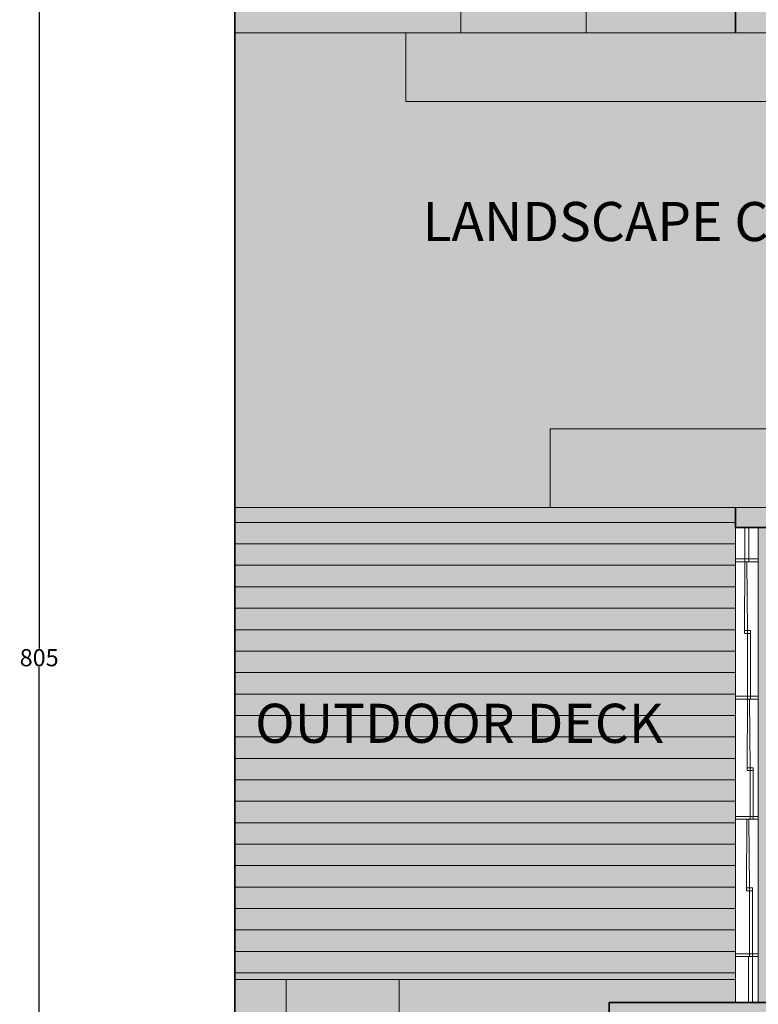
# Model space of a CAD drawing. Units: inches. Extents: x 1704 to 6393, y -157 to 1172.
# Tile 39 of 122: x 1823 to 2081, y 372 to 716. Entities that reach past the tile are written whole.
import ezdxf

# ---------------------------------------------------------------- set-up
doc = ezdxf.new("R2010")
doc.units = ezdxf.units.IN
doc.header["$MEASUREMENT"] = 0
for name, color, linetype, lineweight in [('A-ANNO-DIMS', 7, 'Continuous', 13), ('A-AREA-IDEN', 7, 'Continuous', 18), ('A-WALL-PATT', 7, 'Continuous', 13), ('C-PROP', 7, 'Continuous', 35), ('GLASS PANEL FASADE', 4, 'Continuous', 18), ('L-DECK-PLNK-PATT', 250, 'Continuous', 13), ('L-HRDS', 8, 'Continuous', 18), ('L-PVMT-PATT', 8, 'Continuous', 13), ('WALLS', 7, 'Continuous', 35)]:
    doc.layers.add(name, color=color, linetype=linetype, lineweight=lineweight)
for name, color, linetype, lineweight, true_color in [('A-FLOR-PATT', 7, 'Continuous', 13, 0xf2f2f2), ('L-DECK-PATT', 35, 'Continuous', 13, 0xa6725b), ('L-HRDS-PATT', 9, 'Continuous', 13, 0xc5c1ba), ('L-PLNT-PATT', 253, 'Continuous', 13, 0x9abc8f)]:
    doc.layers.add(name, color=color, linetype=linetype, lineweight=lineweight, true_color=true_color)
doc.styles.get("Standard").update_dxf_attribs({"font": 'arial.ttf'})
doc.dimstyles.get("Standard").update_dxf_attribs({"dimtxt": 6, "dimasz": 2, "dimexe": 0.18, "dimexo": 0.0625, "dimgap": 0.09, "dimtad": 0, "dimtih": 1, "dimtoh": 1, "dimdec": 1, "dimzin": 0, "dimdsep": 46, "dimlunit": 3, "dimtxsty": 'Standard', "dimblk": 'ARCHTICK', "dimcen": 0.09, "dimadec": 0, "dimazin": 0, "dimtfac": 1, "dimtdec": 1, "dimtofl": 0, "dimtmove": 0, "dimatfit": 3, "dimfxl": 1, "dimtolj": 1, "dimtzin": 0, "dimarcsym": 0})

# ---------------------------------------------------------------- blocks, each defined once
blk = doc.blocks.new('_ArchTick')
at = {"color": 0, "linetype": 'ByBlock', "const_width": 0.15}
blk.add_lwpolyline([(-0.5, -0.5), (0.5, 0.5)], dxfattribs=at)
blk = doc.blocks.new('*D93')
at = {"layer": 'A-ANNO-DIMS', "color": 0, "lineweight": -2, "transparency": 16777216}
for p, q in [((2605.29, 895.21), (1829.7, 895.21)), ((1829.88, 895.21), (1829.88, 495.87)), ((1829.88, 90.21), (1829.88, 489.56)), ((2605.29, 90.21), (1829.7, 90.21))]:
    blk.add_line(p, q, dxfattribs=at)
at = {"layer": 'Defpoints', "color": 0, "lineweight": -3, "transparency": 16777216}
for p in [(2605.35, 895.21), (1829.88, 90.21), (2605.35, 90.21)]:
    blk.add_point(p, dxfattribs=at)
at = {"layer": 'A-ANNO-DIMS', "color": 0, "lineweight": -2, "transparency": 16777216, "xscale": 2, "yscale": 2, "zscale": 2}
for p, rotation in [((1829.88, 895.21), 90), ((1829.88, 90.21), 270)]:
    blk.add_blockref('_ArchTick', p, dxfattribs=dict(at, rotation=rotation))
at = {"layer": 'A-ANNO-DIMS', "color": 0, "transparency": 16777216, "insert": (1829.88, 492.71), "char_height": 6, "attachment_point": 5}
blk.add_mtext('\\A1;805', dxfattribs=at)

msp = doc.modelspace()

# ---------------------------------------------------------------- hatches: boundary and pattern name
at = {"layer": 'A-FLOR-PATT', "transparency": 33554528}
h = msp.add_hatch(color=256, dxfattribs=at)
h.dxf.hatch_style = 1
h.paths.add_polyline_path([(2273.349, 538.213), (2081.349, 538.213), (2081.349, 372.213), (2273.349, 372.213)])
h.paths.add_polyline_path([(2189.542, 505.951), (2184.316, 505.951), (2184.316, 505.591), (2169.442, 505.591), (2169.442, 505.951), (2164.216, 505.951, -0.4142136), (2163.814, 506.353), (2163.814, 526.093, -0.4142136), (2164.216, 526.495), (2189.542, 526.495, -0.4142136), (2189.944, 526.093), (2189.944, 506.353, -0.4142136)], flags=16)
h.paths.add_polyline_path([(2200.535, 511.491), (2200.535, 526.191), (2217.621, 526.191), (2217.621, 511.491), (2214.605, 511.491, -0.3946213), (2214.203, 511.116), (2203.952, 511.116, -0.3946213), (2203.551, 511.491)], flags=16)
h.paths.add_polyline_path([(2200.736, 511.692), (2200.736, 525.99), (2203.55, 525.99), (2203.55, 523.838, 0.1045605), (2214.605, 523.838), (2214.605, 525.99), (2217.42, 525.99), (2217.42, 511.692), (2214.605, 511.692), (2214.605, 523.838, -0.1045605), (2203.55, 523.838), (2203.55, 511.692)], flags=0)
h.paths.add_polyline_path([(2203.952, 511.317, -0.4142136), (2203.751, 511.518), (2203.751, 523.591, 0.099912), (2214.404, 523.591), (2214.404, 511.518, -0.4142136), (2214.203, 511.317)], flags=0)
h.paths.add_polyline_path([(2184.084, 516.015, -0.0686795), (2169.674, 516.015), (2169.674, 522.073), (2184.084, 522.073)], flags=0)
h.paths.add_polyline_path([(2183.325, 518.606, -0.0772766), (2170.433, 518.606), (2170.433, 521.123, -0.0235462), (2183.325, 521.123)], flags=0)
h.paths.add_polyline_path([(2135.029, 507.225, -0.1405189), (2135.191, 507.834, -0.0513838), (2135.029, 507.797)], flags=16)
h.paths.add_polyline_path([(2146.318, 498.997, -0.0311848), (2144.279, 499.202, -0.1719602), (2141.865, 499.263, -0.2234326), (2139.482, 499.263, -0.1719602), (2137.068, 499.202, -0.0311848), (2135.029, 498.997, -0.066975), (2135.029, 505.313, -0.0276914), (2136.841, 505.144), (2136.841, 506.777), (2136.576, 506.777), (2136.576, 507.371, 0.039911), (2145.741, 507.448, 0.2546956), (2146.318, 507.225), (2146.318, 507.269, 0.1305786), (2146.156, 507.834, -0.0704067), (2145.953, 507.935, -0.011584), (2145.714, 508.002, -0.2546956), (2145.137, 507.779, -0.2546956), (2145.361, 508.355, -0.0259693), (2145.107, 516.407, -0.0070422), (2144.025, 516.297, -0.1828112), (2142.939, 516.218, -0.2042746), (2142.015, 516.175, -0.1805419), (2139.348, 516.174, -0.0000184), (2139.345, 516.174, -0.2035615), (2138.425, 516.217, -0.0000237), (2138.421, 516.217, -0.1818152), (2137.34, 516.296, -0.0071635), (2136.24, 516.407, 0.007166), (2136.162, 518.63, 0.314303), (2135.854, 518.974, -0.1253469), (2135.537, 518.935, -0.2546956), (2135.76, 519.512, -0.0162662), (2135.67, 519.849, -0.296972), (2135.535, 520.8, -0.227702), (2135.464, 521.698, 0.1283977), (2132.757, 521.718), (2132.757, 525.785, -0.4142136), (2133.331, 526.359), (2148.015, 526.359, -0.4142136), (2148.589, 525.785), (2148.589, 521.718, -0.0118936), (2148.835, 521.65, -0.2546956), (2149.412, 521.873, -0.2546956), (2149.188, 521.296, -0.0417628), (2149.188, 508.355, -0.2546956), (2149.412, 507.779, -0.2546956), (2148.835, 508.002, -0.011584), (2148.596, 507.935, -0.2124435), (2147.949, 507.813, -0.2363999), (2147.423, 507.772, -0.3143526), (2147.126, 507.772, -0.2363999), (2146.6, 507.813, -0.0879275), (2146.318, 507.797), (2146.318, 507.225, -0.2546956), (2145.741, 507.448, -0.0042329), (2144.771, 507.371), (2144.771, 506.777), (2144.506, 506.777), (2144.506, 505.144, -0.0276914), (2146.318, 505.313, -0.066975)], flags=16)
h.paths.add_polyline_path([(2141.865, 505.047, 0.2234326), (2139.482, 505.047, 0.1738145), (2137.043, 505.1), (2137.043, 506.317), (2137.335, 506.317), (2137.335, 505.184, -0.1522072), (2139.482, 505.047, -0.2234326), (2141.865, 505.047, -0.1522072), (2144.011, 505.184), (2144.011, 506.317), (2144.304, 506.317), (2144.304, 505.1, 0.1738145)], flags=0)
h.paths.add_polyline_path([(2145.233, 522.986, 0.0079197), (2144.017, 523.111, 0.1826165), (2142.931, 523.19, 0.2042746), (2142.008, 523.233, 0.1806536), (2139.339, 523.233, 0.2042746), (2138.415, 523.19, 0.1826165), (2137.33, 523.111, 0.0079197), (2136.114, 522.986, 0.1967082), (2135.679, 523.212, 0.047677), (2135.755, 524.004), (2134.638, 521.852), (2134.376, 524.691, -0.2583282), (2135.029, 526.359, -0.0890464), (2135.632, 525.01, -0.1830277), (2145.715, 525.01, -0.0890464), (2146.318, 526.359, -0.2583282), (2146.971, 524.691), (2146.709, 521.852), (2145.592, 524.004, 0.047677), (2145.668, 523.212, 0.1967082)], flags=0)
h.paths.add_polyline_path([(2144.419, 519.027, -0.0368796), (2136.927, 519.027, -0.0368796)], flags=0)
h.paths.add_polyline_path([(2273.349, 629.213), (2213.349, 629.213), (2213.349, 573.213), (2213.349, 545.213), (2273.349, 545.213)])
h.paths.add_polyline_path([(2273.349, 711.213), (2207.349, 711.213), (2207.349, 709.213), (2231.349, 709.213), (2231.349, 707.213), (2207.349, 707.213), (2207.349, 631.213), (2273.349, 631.213)])
h.paths.add_polyline_path([(2273.349, 364.213), (2081.349, 364.213), (2081.349, 202.213), (2225.349, 202.213), (2229.181, 202.213), (2230.482, 202.213), (2268.215, 202.213), (2269.516, 202.213), (2273.349, 202.213)])
h.paths.add_polyline_path([(2203.551, 339.558, 0.3946213), (2203.952, 339.183), (2214.203, 339.183), (2214.203, 339.384), (2203.751, 339.384), (2203.751, 339.558)], flags=16)
h.paths.add_polyline_path([(2203.55, 351.7), (2203.55, 339.759), (2200.535, 339.759), (2200.535, 354.258), (2217.621, 354.258), (2217.621, 339.558), (2214.404, 339.558), (2214.404, 351.659, -0.101837)], flags=16)
h.paths.add_polyline_path([(2214.404, 354.057), (2214.605, 354.057), (2214.605, 354.258), (2214.404, 354.258)], flags=16)
h.paths.add_polyline_path([(2189.542, 334.018), (2184.316, 334.018), (2184.316, 333.658), (2169.442, 333.658), (2169.442, 334.018), (2164.216, 334.018, -0.4142136), (2163.814, 334.42), (2163.814, 354.161, -0.4142136), (2164.216, 354.563), (2189.542, 354.563, -0.4142136), (2189.944, 354.161), (2189.944, 334.42, -0.4142136)], flags=16)
h.paths.add_polyline_path([(2184.084, 344.083, -0.0686795), (2169.674, 344.083), (2169.674, 349.85), (2165.7, 350.14), (2188.058, 350.14), (2184.084, 349.85)], flags=0)
h.paths.add_polyline_path([(2183.325, 346.673, -0.0772766), (2170.433, 346.673), (2170.433, 349.19, -0.0235462), (2183.325, 349.19)], flags=0)
h.paths.add_polyline_path([(2134.638, 349.919), (2134.376, 352.758, -0.2583282), (2135.029, 354.426), (2133.331, 354.426, 0.4142136), (2132.757, 353.852), (2132.757, 349.785, -0.0886664)], flags=16)
h.paths.add_polyline_path([(2136.114, 351.053, -0.0079197), (2137.33, 351.178, -0.1826165), (2138.415, 351.257, -0.2042746), (2139.339, 351.3, -0.1806536), (2142.008, 351.3, -0.2042746), (2142.931, 351.257, -0.1826165), (2144.017, 351.178, -0.0079197), (2145.233, 351.053, -0.1967082), (2145.668, 351.279, -0.047677), (2145.592, 352.071, 0.1133241), (2135.755, 352.071, -0.047677), (2135.679, 351.279, -0.1967082)], flags=16)
h.paths.add_polyline_path([(2145.184, 346.697, 0.0331414), (2145.361, 336.423, 0.2546956), (2145.137, 335.846, 0.3030408), (2145.781, 336.164, 0.2903634), (2146.6, 335.88, 0.2363999), (2147.126, 335.839, -0.280712), (2147.275, 336.69, -0.280712), (2147.423, 335.839, 0.2363999), (2147.949, 335.88, 0.2903634), (2148.768, 336.164, 0.3030408), (2149.412, 335.846, 0.2546956), (2149.188, 336.423, 0.0417628), (2149.188, 349.363, 0.2546956), (2149.412, 349.94, 0.2546956), (2148.835, 349.717, 0.1405058), (2145.883, 349.765, -0.227702), (2145.812, 348.867, -0.296972), (2145.677, 347.916, -0.0162662), (2145.586, 347.579, -0.2546956), (2145.81, 347.002, -0.1253469), (2145.493, 347.041, 0.314303)], flags=16)
h.paths.add_polyline_path([(2135.029, 335.292, -0.1405189), (2135.191, 335.901, -0.1399435), (2134.747, 335.88, -0.2363999), (2134.22, 335.839, -0.3143526), (2133.924, 335.839, -0.280712), (2134.072, 336.69, -0.280712), (2134.22, 335.839, 0.2363999), (2134.747, 335.88, 0.2903634), (2135.566, 336.164, 0.3030408), (2136.209, 335.846, 0.2546956), (2135.985, 336.423, 0.0331414), (2136.162, 346.697, 0.314303), (2135.854, 347.041, -0.1253469), (2135.537, 347.002, -0.2546956), (2135.76, 347.579, -0.0162662), (2135.67, 347.916, -0.296972), (2135.535, 348.867, -0.2999866), (2135.599, 350.01, -0.0330719), (2135.76, 350.7, -0.3502076), (2135.604, 351.492), (2134.638, 349.919), (2135.604, 351.492, 0.3502076), (2135.76, 350.7, 0.0330719), (2135.599, 350.01, 0.2999866), (2135.535, 348.867, 0.296972), (2135.67, 347.916, 0.0279375), (2135.971, 347.698, 0.3576436), (2135.537, 347.002, 0.1253469), (2135.854, 347.041, -0.3555912), (2136.165, 346.637, -0.0329482), (2135.985, 336.423, -0.2546956), (2136.209, 335.846, -0.2546956), (2135.632, 336.069, -0.011584), (2135.393, 336.003, -0.1222327), (2135.029, 335.864)], flags=16)
h.paths.add_polyline_path([(2136.841, 335.42), (2136.783, 335.423), (2136.783, 334.844), (2136.841, 334.471)], flags=16)
h.paths.add_polyline_path([(2146.318, 327.064, -0.0311848), (2144.279, 327.269, -0.1719602), (2141.865, 327.33, -0.2234326), (2139.482, 327.33, -0.1719602), (2137.068, 327.269, -0.0311848), (2135.029, 327.064, -0.066975), (2135.029, 333.38, -0.0311848), (2137.068, 333.175, -0.1719602), (2139.482, 333.114, -0.2234326), (2141.865, 333.114, -0.1522072), (2144.011, 333.251), (2144.011, 334.384), (2144.304, 335.406, 0.0020345), (2144.771, 335.438), (2144.771, 334.844), (2144.506, 333.211, -0.0276914), (2146.318, 333.38, -0.066975)], flags=16)
h.paths.add_polyline_path([(2137.129, 334.384), (2137.335, 334.384), (2137.335, 333.251), (2137.129, 333.195)], flags=16)
h.paths.add_polyline_path([(2144.419, 347.094, -0.0368796), (2136.927, 347.094, -0.0368796)], flags=16)
at = {"layer": 'A-WALL-PATT', "transparency": 33554643}
h = msp.add_hatch(color=256, dxfattribs=at)
h.dxf.hatch_style = 1
h.paths.add_polyline_path([(2167.349, 895.213), (2073.349, 895.213), (2073.349, 887.213), (2081.349, 887.213), (2167.349, 887.213)])
h.paths.add_polyline_path([(2465.349, 895.213), (2273.349, 895.213), (2273.349, 903.213), (2263.349, 903.213), (2263.349, 895.213), (2263.349, 887.213), (2325.349, 887.213), (2325.349, 863.213), (2333.349, 863.213), (2333.349, 887.213), (2465.349, 887.213)])
h.paths.add_polyline_path([(2533.349, 895.213), (2513.349, 895.213), (2513.349, 887.213), (2513.349, 861.213), (2517.349, 861.213), (2517.349, 887.213), (2533.349, 887.213)])
h.paths.add_polyline_path([(2605.349, 895.213), (2581.349, 895.213), (2581.349, 887.213), (2597.349, 887.213), (2597.349, 854.213), (2605.349, 854.213)])
h.paths.add_polyline_path([(2605.349, 752.213), (2629.349, 752.213), (2629.349, 716.213), (2605.349, 716.213), (2605.349, 712.213), (2719.349, 712.213), (2719.349, 716.213), (2631.349, 716.213), (2631.349, 754.213), (2605.349, 754.213), (2605.349, 794.213), (2597.349, 794.213), (2597.349, 787.213), (2517.349, 787.213), (2517.349, 813.213), (2513.349, 813.213), (2513.349, 783.213), (2517.349, 783.213), (2597.349, 783.213), (2597.349, 719.213), (2517.349, 719.213), (2517.349, 753.213), (2513.349, 753.213), (2513.349, 719.213), (2365.349, 719.213), (2365.349, 763.213), (2325.349, 763.213), (2325.349, 755.213), (2357.349, 755.213), (2357.349, 719.213), (2325.349, 719.213), (2325.349, 711.213), (2547.349, 711.213), (2547.349, 615.213), (2449.349, 615.213), (2449.349, 607.213), (2514.349, 607.213), (2514.349, 546.213), (2439.349, 546.213), (2425.349, 546.213), (2425.349, 607.213), (2425.349, 615.213), (2350.349, 615.213), (2350.349, 589.713), (2358.349, 589.713), (2358.349, 610.213), (2420.349, 610.213), (2420.349, 545.213), (2358.349, 545.213), (2358.349, 565.713), (2350.349, 565.713), (2350.349, 538.213), (2469.349, 538.213), (2469.349, 459.213), (2469.349, 372.213), (2423.349, 372.213), (2423.349, 364.213), (2473.349, 364.213), (2473.349, 318.213), (2477.349, 318.213), (2477.349, 364.213), (2547.349, 364.213), (2547.349, 352.213), (2549.349, 352.213), (2549.349, 364.213), (2597.349, 364.213), (2597.349, 328.213), (2549.349, 328.213), (2547.349, 328.213), (2547.349, 326.213), (2549.349, 326.213), (2597.349, 326.213), (2605.349, 326.213), (2605.349, 377.057), (2597.349, 377.057), (2597.349, 372.213), (2477.349, 372.213), (2477.349, 451.213), (2597.349, 451.213), (2605.349, 451.213), (2605.349, 459.213), (2597.349, 459.213), (2477.349, 459.213), (2477.349, 538.213), (2597.349, 538.213), (2597.349, 495.213), (2605.349, 495.213), (2605.349, 512.213), (2631.349, 512.213), (2631.349, 568.213), (2605.349, 568.213), (2605.349, 577.213), (2597.349, 577.213), (2597.349, 542.213), (2518.349, 542.213), (2518.349, 607.213), (2532.349, 607.213), (2605.349, 607.213), (2605.349, 615.213), (2597.349, 615.213), (2551.349, 615.213), (2551.349, 711.213), (2597.349, 711.213), (2597.349, 645.213), (2605.349, 645.213), (2605.349, 712.213), (2605.349, 716.213)])
h.paths.add_polyline_path([(2605.349, 566.213), (2629.349, 566.213), (2629.349, 514.213), (2605.349, 514.213)], flags=16)
h.paths.add_polyline_path([(2381.349, 372.213), (2349.349, 372.213), (2349.349, 202.213), (2337.349, 202.213), (2337.349, 194.213), (2349.349, 194.213), (2349.349, 90.213), (2349.349, 72.213), (2357.349, 72.213), (2357.349, 90.213), (2381.349, 90.213), (2381.349, 98.213), (2357.349, 98.213), (2357.349, 266.213), (2381.349, 266.213), (2381.349, 270.213), (2353.349, 270.213), (2353.349, 364.213), (2381.349, 364.213)])
h.paths.add_polyline_path([(2605.349, 302.213), (2597.349, 302.213), (2597.349, 270.213), (2477.349, 270.213), (2477.349, 294.213), (2473.349, 294.213), (2473.349, 270.213), (2423.349, 270.213), (2423.349, 266.213), (2597.349, 266.213), (2597.349, 218.213), (2605.349, 218.213)])
h.paths.add_polyline_path([(2605.349, 146.213), (2597.349, 146.213), (2597.349, 98.213), (2429.349, 98.213), (2429.349, 90.213), (2597.349, 90.213), (2597.349, 72.213), (2605.349, 72.213), (2605.349, 90.213)])
h.paths.add_polyline_path([(2225.349, 202.213), (2049.349, 202.213), (2049.349, 194.213), (2225.349, 194.213)])
h.paths.add_polyline_path([(2289.349, 202.213), (2277.349, 202.213), (2273.349, 202.213), (2269.516, 202.213), (2269.516, 194.213), (2273.349, 194.213), (2277.349, 194.213), (2289.349, 194.213)])
h.paths.add_polyline_path([(2273.349, 372.213), (2029.19, 372.213), (2029.19, 364.213), (2273.349, 364.213)])
h.paths.add_polyline_path([(2277.349, 545.213), (2213.349, 545.213), (2213.349, 573.213), (2205.349, 573.213), (2177.349, 573.213), (2177.349, 545.213), (2073.349, 545.213), (2073.349, 538.213), (2081.349, 538.213), (2277.349, 538.213)])
h.paths.add_polyline_path([(2181.349, 545.213), (2181.349, 569.213), (2205.349, 569.213), (2205.349, 545.213)], flags=16)
h.paths.add_polyline_path([(2277.349, 719.213), (2081.349, 719.213), (2073.349, 719.213), (2073.349, 711.213), (2154.575, 711.213), (2205.349, 711.213), (2205.349, 687.213), (2205.349, 629.213), (2213.349, 629.213), (2273.349, 629.213), (2273.349, 631.213), (2207.349, 631.213), (2207.349, 707.213), (2231.349, 707.213), (2231.349, 709.213), (2207.349, 709.213), (2207.349, 711.213), (2277.349, 711.213)])
at = {"layer": 'L-DECK-PATT', "transparency": 33554592}
h = msp.add_hatch(color=256, dxfattribs=at)
h.dxf.hatch_style = 1
h.paths.add_polyline_path([(2073.349, 538.213), (2073.349, 545.213), (1898.349, 545.213), (1898.349, 380.213), (2073.349, 380.213)])
at = {"layer": 'L-DECK-PLNK-PATT'}
h = msp.add_hatch(dxfattribs=at)
h.set_pattern_fill('LINE', color=256, scale=60)
h.paths.add_polyline_path([(2073.349, 538.213), (2073.349, 545.213), (1898.349, 545.213), (1898.349, 380.213), (2073.349, 380.213)])
at = {"layer": 'L-HRDS-PATT', "transparency": 33554643}
h = msp.add_hatch(color=256, dxfattribs=at)
h.dxf.hatch_style = 1
h.paths.add_polyline_path([(2073.349, 719.213), (2021.151, 719.213), (2021.151, 711.213), (2073.349, 711.213)])
h.paths.add_polyline_path([(1977.349, 719.213), (1969.349, 719.213), (1898.349, 719.213), (1898.349, 711.213), (1977.349, 711.213)])
h.paths.add_polyline_path([(1977.349, 895.213), (1898.349, 895.213), (1898.349, 887.213), (1969.349, 887.213), (1977.349, 887.213)])
h = msp.add_hatch(color=256, dxfattribs=at)
h.dxf.hatch_style = 1
h.paths.add_polyline_path([(2154.575, 711.213), (1958.127, 711.213), (1958.127, 687.213), (2154.575, 687.213)])
h.paths.add_polyline_path([(2205.349, 711.213), (2159.484, 711.213), (2159.484, 687.213), (2205.349, 687.213)])
h.paths.add_polyline_path([(2177.349, 572.777), (2008.58, 572.777), (2008.58, 545.213), (2177.349, 545.213)])
h = msp.add_hatch(color=256, dxfattribs=at)
h.dxf.hatch_style = 1
h.paths.add_polyline_path([(1955.732, 380.213), (1916.214, 380.213), (1916.214, 325.779), (1955.732, 325.779)])
h.paths.add_polyline_path([(1955.732, 318.405), (1916.214, 318.405), (1916.214, 279.355), (1955.732, 279.355)])
h.paths.add_polyline_path([(1955.732, 270.314), (1916.214, 270.314), (1916.214, 234.313), (1955.732, 234.313)])
h.paths.add_polyline_path([(2073.349, 230.029), (1898.349, 230.029), (1898.349, 202.213), (2073.349, 202.213)])
at = {"layer": 'L-PLNT-PATT', "transparency": 33554643}
h = msp.add_hatch(color=256, dxfattribs=at)
h.dxf.hatch_style = 1
h.paths.add_polyline_path([(2205.349, 687.213), (2159.484, 687.213), (2159.484, 711.213), (2154.575, 711.213), (2154.575, 687.213), (1958.127, 687.213), (1958.127, 711.213), (1898.349, 711.213), (1898.349, 545.213), (2008.58, 545.213), (2008.58, 572.777), (2177.349, 572.777), (2177.349, 573.213), (2205.349, 573.213), (2205.349, 629.213)])
h = msp.add_hatch(color=256, dxfattribs=at)
h.dxf.hatch_style = 1
h.paths.add_polyline_path([(2073.349, 364.213), (2029.19, 364.213), (2029.19, 372.213), (2073.349, 372.213), (2073.349, 380.213), (1955.732, 380.213), (1955.732, 325.779), (1916.214, 325.779), (1916.214, 380.213), (1898.349, 380.213), (1898.349, 230.029), (2073.349, 230.029)])
h.paths.add_polyline_path([(1955.732, 279.355), (1916.214, 279.355), (1916.214, 318.405), (1955.732, 318.405)], flags=16)
h.paths.add_polyline_path([(1955.732, 270.314), (1955.732, 234.313), (1916.214, 234.313), (1916.214, 270.314)], flags=16)
at = {"layer": 'L-PVMT-PATT'}
h = msp.add_hatch(dxfattribs=at)
h.set_pattern_fill('GRAVEL', color=256, scale=4)
h.set_pattern_definition([(228.012788, (2.88, 4), (-32, -36), [0.538144, -53.276352]), (184.969741, (2.52, 3.6), (48, 4), [0.923472, -91.423699]), (132.510447, (1.6, 3.52), (40, -44), [0.651152, -64.4641304]), (267.273689, (0.04, 2.52), (4, 80), [0.840952, -83.254232]), (292.833654, (0, 1.68), (-20, 48), [0.82462, -81.6374925]), (357.273689, (0.32, 0.92), (-80, 4), [0.840952, -83.254232]), (37.6942405, (1.16, 0.88), (-52, -40), [1.112116, -110.099394]), (72.255328, (2.04, 1.56), (28, 88), [1.049952, -103.945286]), (121.429566, (2.36, 2.56), (-32, 52), [0.8438, -83.5362924]), (175.236358, (1.92, 3.28), (44, -4), [0.963328, -47.20305]), (222.397438, (0.96, 3.36), (-48, -44), [1.245792, -123.3335]), (138.814075, (4, 2.48), (-28, 24), [0.425204, -42.095379]), (171.469234, (3.68, 2.76), (52, -8), [0.808948, -80.086046]), (225, (2.88, 2.88), (-4e-16, -4), [0.565684, -5.09117]), (203.19859, (2.6, 3.36), (20, 8), [0.304632, -30.1584604]), (291.80141, (2.32, 3.24), (-4, 12), [0.430812, -21.109847]), (30.963757, (2.48, 2.84), (12, 8), [0.699716, -22.6240916]), (161.56505, (3.08, 3.2), (8, -4), [0.505964, -12.143147]), (16.38954, (0, 3.24), (40, 12), [0.7088, -70.1713806]), (70.346176, (0.68, 3.44), (-16, -44), [0.594644, -58.869631]), (293.19859, (3.08, 4), (-8, 20), [0.60926, -29.8538324]), (343.61046, (3.32, 3.44), (-40, 12), [0.7088, -70.1713806]), (339.443955, (0, 0.76), (-20, 8), [0.68352, -33.492495]), (294.77514, (0.64, 0.52), (-20, 44), [0.572712, -56.698572]), (66.80141, (3.12, 0), (8, 20), [0.60926, -29.8538324]), (17.354025, (3.36, 0.56), (-52, -16), [0.670524, -66.3816945]), (69.443955, (1.16, 0), (-8, -20), [0.34176, -33.834255]), (101.309932, (2.88, 0), (-4, 16), [0.20396, -20.192118]), (165.963757, (2.84, 0.2), (12, -4), [0.82462, -15.6678025]), (186.009006, (2.04, 0.4), (40, 4), [0.7642, -75.655693]), (303.69007, (2.48, 2.48), (-4, 8), [0.576888, -13.845317]), (353.1572266, (2.8, 2), (68, -8), [1.007176, -99.7102505]), (60.945396, (3.8, 1.88), (-16, -28), [0.411824, -40.7706966]), (90, (4, 2.24), (-4, 4), [0.24, -3.76]), (120.256437, (1.96, 0.52), (16, -28), [0.555696, -55.01408]), (48.012788, (1.68, 1), (32, 36), [1.076288, -52.738208]), (0, (2.4, 1.8), (4, 4), [1.04, -2.96]), (325.304846, (3.44, 1.8), (40, -28), [0.632456, -62.613097]), (254.054604, (3.96, 1.44), (-4, -16), [0.582408, -28.5380316]), (207.645975, (3.8, 0.88), (-76, -40), [0.94826, -93.877897]), (175.426079, (2.96, 0.44), (-52, 4), [1.003196, -99.3162936])])
h.paths.add_polyline_path([(1977.349, 887.213), (1969.349, 887.213), (1969.349, 719.213), (1977.349, 719.213)])
h.paths.add_polyline_path([(2021.151, 895.213), (1977.349, 895.213), (1977.349, 887.213), (2021.151, 887.213)])
h.paths.add_polyline_path([(2021.151, 719.213), (1977.349, 719.213), (1977.349, 711.213), (2021.151, 711.213)])

# ---------------------------------------------------------------- linework, layer by layer
at = {"layer": 'C-PROP'}
msp.add_line((1898.349, -3.787), (1898.349, 1033.213), dxfattribs=at)
at = {"layer": 'GLASS PANEL FASADE'}
for p, q in [((2073.349, 372.213), (2073.349, 538.213)), ((2073.349, 538.213), (2081.349, 538.213)), ((2076.649, 526.213), (2076.649, 538.213)), ((2078.049, 526.213), (2078.049, 538.213)), ((2081.349, 538.213), (2081.349, 372.213)), ((2073.349, 527.213), (2081.349, 527.213)), ((2073.349, 526.213), (2081.349, 526.213)), ((2076.57, 502.214), (2076.649, 526.213)), ((2077.349, 526.213), (2077.57, 502.214)), ((2077.57, 502.214), (2076.57, 502.214)), ((2076.57, 502.214), (2076.57, 501.214)), ((2076.57, 501.214), (2078.57, 501.214)), ((2077.57, 502.214), (2078.57, 502.214)), ((2077.57, 502.214), (2077.57, 478.213)), ((2078.57, 502.214), (2078.57, 478.213)), ((2073.349, 479.213), (2081.349, 479.213)), ((2073.349, 478.213), (2081.349, 478.213)), ((2077.492, 454.214), (2077.57, 478.213)), ((2078.27, 478.213), (2078.492, 454.214)), ((2078.492, 454.214), (2077.492, 454.214)), ((2077.492, 454.214), (2077.492, 453.214)), ((2077.492, 453.214), (2079.492, 453.214)), ((2078.492, 454.214), (2079.492, 454.214)), ((2078.492, 454.214), (2078.492, 436.213)), ((2079.492, 454.214), (2079.492, 436.213)), ((2081.349, 437.213), (2073.349, 437.213)), ((2081.349, 436.213), (2073.349, 436.213)), ((2077.27, 412.214), (2077.349, 436.213)), ((2078.049, 436.213), (2078.27, 412.214)), ((2078.27, 412.214), (2077.27, 412.214)), ((2077.27, 412.214), (2077.27, 411.214)), ((2077.27, 411.214), (2079.27, 411.214)), ((2078.27, 412.214), (2079.27, 412.214)), ((2078.27, 412.214), (2078.27, 388.213)), ((2079.27, 412.214), (2079.27, 388.213)), ((2081.349, 389.213), (2073.349, 389.213)), ((2081.349, 388.213), (2073.349, 388.213)), ((2077.87, 388.213), (2077.87, 372.213)), ((2079.27, 388.213), (2079.27, 372.213)), ((2081.349, 372.213), (2073.349, 372.213))]:
    msp.add_line(p, q, dxfattribs=at)
at = {"layer": 'L-HRDS'}
for p, q in [((1977.349, 719.213), (1977.349, 711.213)), ((2021.151, 719.213), (2021.151, 711.213)), ((2205.349, 711.213), (1898.349, 711.213)), ((2073.349, 545.213), (1898.349, 545.213)), ((2177.349, 545.213), (2073.349, 545.213)), ((2073.349, 380.213), (1898.349, 380.213))]:
    msp.add_line(p, q, dxfattribs=at)
for points in [[(2154.575, 711.213), (1958.127, 711.213), (1958.127, 687.213), (2154.575, 687.213)], [(2177.349, 545.213), (2008.58, 545.213), (2008.58, 572.777), (2177.349, 572.777)], [(1916.214, 380.213), (1955.732, 380.213), (1955.732, 325.779), (1916.214, 325.779)]]:
    msp.add_lwpolyline(points, close=True, dxfattribs=at)
at = {"layer": 'WALLS'}
for p, q in [((2073.349, 719.213), (2073.349, 711.213)), ((2073.349, 538.213), (2073.349, 545.213)), ((2081.349, 538.213), (2073.349, 538.213)), ((2277.349, 538.213), (2081.349, 538.213)), ((2277.349, 372.213), (2029.19, 372.213)), ((2029.19, 364.213), (2029.19, 372.213))]:
    msp.add_line(p, q, dxfattribs=at)

# ---------------------------------------------------------------- texts
at = {"layer": 'A-AREA-IDEN'}
for s, p in [('LANDSCAPE COURT', (1963.906, 638.365)), ('OUTDOOR DECK', (1905.394, 462.932))]:
    msp.add_text(s, height=13.6672, dxfattribs=at).set_placement(p)

# ---------------------------------------------------------------- dimensions: what is measured, and where the dimension line sits
at = {"layer": 'A-ANNO-DIMS'}
dim = msp.add_linear_dim(base=(1829.878, 90.213), p1=(2605.349, 895.213), p2=(2605.349, 90.213), angle=90, dimstyle='Standard', override={"dimdec": 0, "dimlfac": 1, "dimrnd": 0, "dimzin": 0, "dimdsep": 46, "dimlunit": 2}, dxfattribs=at)
dim.commit()
dim.dimension.update_dxf_attribs({"geometry": '*D93', "text_midpoint": (1829.878, 492.713)})

doc.saveas('drawing.dxf')
